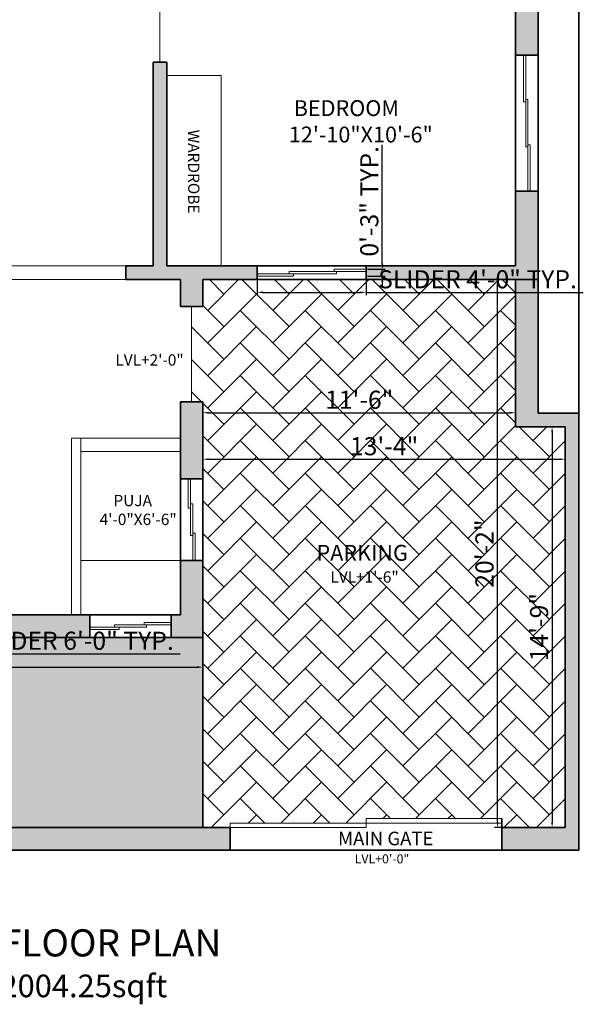
# Model space of a CAD drawing. Units: inches. Extents: x 3491 to 6898, y 1360 to 2019.
# Tile 2 of 9: x 3825 to 4074, y 1360 to 1795. Entities that reach past the tile are written whole.
import ezdxf

# ---------------------------------------------------------------- set-up
doc = ezdxf.new("R2010")
doc.units = ezdxf.units.IN
for name, color, linetype, lineweight in [('A-ANNO-DIMS', 2, 'Continuous', 18), ('A-ANNO-TEXT', 7, 'Continuous', 18), ('A-ANNO-TITL', 7, 'Continuous', 30), ('A-AREA-IDEN', 7, 'Continuous', 18), ('A-DOOR', 4, 'Continuous', 18), ('A-FLOR-CASE', 8, 'Continuous', 18), ('A-FLOR-PATT', 252, 'Continuous', 13), ('A-GLAZ', 5, 'Continuous', 18), ('A-WALL', 7, 'Continuous', 35), ('A-WALL-PATT', 8, 'Continuous', 13)]:
    doc.layers.add(name, color=color, linetype=linetype, lineweight=lineweight)
doc.layers.add('A-WALL-OPEN', color=251, linetype='Continuous', lineweight=13, true_color=0x636466)
doc.styles.get("Standard").update_dxf_attribs({"font": 'arial.ttf'})
doc.dimstyles.new('ISO-25', dxfattribs={"dimtxt": 8, "dimasz": 2.5, "dimexe": 1.25, "dimexo": 0.625, "dimtad": 1, "dimdec": 1, "dimlunit": 3, "dimtxsty": 'Standard', "dimcen": 2.5, "dimclrt": 1, "dimadec": 0, "dimazin": 0, "dimtfac": 1, "dimtdec": 1, "dimtmove": 0, "dimatfit": 3, "dimfxl": 1, "dimarcsym": 0})

# ---------------------------------------------------------------- blocks, each defined once
blk = doc.blocks.new('*D8')
at = {"layer": 'A-ANNO-DIMS', "color": 0, "lineweight": -2, "transparency": 16777216}
for p, q in [((3906.13, 1521.74), (3906.13, 1507.99)), ((3674.13, 1515.52), (3674.13, 1507.99)), ((3676.63, 1509.24), (3903.63, 1509.24))]:
    blk.add_line(p, q, dxfattribs=at)
at = {"layer": 'A-ANNO-DIMS', "color": 0, "transparency": 16777216}
for points in [[(3676.63, 1509.66), (3676.63, 1508.83), (3674.13, 1509.24)], [(3903.63, 1509.66), (3903.63, 1508.83), (3906.13, 1509.24)]]:
    blk.add_solid(points, dxfattribs=at)
at = {"layer": 'Defpoints', "color": 0, "transparency": 16777216}
for p in [(3906.13, 1522.37), (3674.13, 1516.15), (3906.13, 1509.24)]:
    blk.add_point(p, dxfattribs=at)
at = {"layer": 'A-ANNO-DIMS', "color": 0, "transparency": 16777216, "insert": (3790.13, 1513.95), "char_height": 8, "attachment_point": 5}
blk.add_mtext('19\'-4"', dxfattribs=at)
blk = doc.blocks.new('*D25')
at = {"layer": 'A-ANNO-DIMS', "color": 0, "lineweight": -2, "transparency": 16777216}
for p, q in [((3906.13, 1617.55), (3906.13, 1622.78)), ((3908.63, 1621.53), (4041.63, 1621.53)), ((4044.13, 1617.55), (4044.13, 1622.78))]:
    blk.add_line(p, q, dxfattribs=at)
at = {"layer": 'A-ANNO-DIMS', "color": 0, "transparency": 16777216}
for points in [[(3908.63, 1621.95), (3908.63, 1621.12), (3906.13, 1621.53)], [(4041.63, 1621.95), (4041.63, 1621.12), (4044.13, 1621.53)]]:
    blk.add_solid(points, dxfattribs=at)
at = {"layer": 'Defpoints', "color": 0, "transparency": 16777216}
for p in [(4044.13, 1621.53), (3906.13, 1616.92), (4044.13, 1616.92)]:
    blk.add_point(p, dxfattribs=at)
at = {"layer": 'A-ANNO-DIMS', "color": 0, "transparency": 16777216, "insert": (3975.13, 1626.24), "char_height": 8, "attachment_point": 5}
blk.add_mtext('11\'-6"', dxfattribs=at)
blk = doc.blocks.new('*D26')
at = {"layer": 'A-ANNO-DIMS', "color": 0, "lineweight": -2, "transparency": 16777216}
for p, q in [((3906.13, 1601.63), (3906.13, 1602.25)), ((3908.63, 1601), (4063.63, 1601)), ((4066.13, 1601.63), (4066.13, 1602.25))]:
    blk.add_line(p, q, dxfattribs=at)
at = {"layer": 'A-ANNO-DIMS', "color": 0, "transparency": 16777216}
for points in [[(3908.63, 1601.42), (3908.63, 1600.59), (3906.13, 1601)], [(4063.63, 1601.42), (4063.63, 1600.59), (4066.13, 1601)]]:
    blk.add_solid(points, dxfattribs=at)
at = {"layer": 'Defpoints', "color": 0, "transparency": 16777216}
for p in [(3906.13, 1601), (4066.13, 1601), (4066.13, 1601)]:
    blk.add_point(p, dxfattribs=at)
at = {"layer": 'A-ANNO-DIMS', "color": 0, "transparency": 16777216, "insert": (3986.13, 1605.72), "char_height": 8, "attachment_point": 5}
blk.add_mtext('13\'-4"', dxfattribs=at)
blk = doc.blocks.new('*D27')
at = {"layer": 'A-ANNO-DIMS', "color": 0, "lineweight": -2, "transparency": 16777216}
for p, q in [((4065.51, 1615.37), (4059.06, 1615.37)), ((4060.31, 1612.87), (4060.31, 1440.87)), ((4065.51, 1438.37), (4059.06, 1438.37))]:
    blk.add_line(p, q, dxfattribs=at)
at = {"layer": 'A-ANNO-DIMS', "color": 0, "transparency": 16777216}
for points in [[(4059.89, 1612.87), (4060.73, 1612.87), (4060.31, 1615.37)], [(4059.89, 1440.87), (4060.73, 1440.87), (4060.31, 1438.37)]]:
    blk.add_solid(points, dxfattribs=at)
at = {"layer": 'Defpoints', "color": 0, "transparency": 16777216}
for p in [(4066.13, 1615.37), (4060.31, 1438.37), (4066.13, 1438.37)]:
    blk.add_point(p, dxfattribs=at)
at = {"layer": 'A-ANNO-DIMS', "color": 0, "transparency": 16777216, "insert": (4055.6, 1526.87), "char_height": 8, "attachment_point": 5, "rotation": 90}
blk.add_mtext('14\'-9"', dxfattribs=at)
blk = doc.blocks.new('*D28')
at = {"layer": 'A-ANNO-DIMS', "color": 0, "lineweight": -2, "transparency": 16777216}
for p, q in [((4043.51, 1680.37), (4034.93, 1680.37)), ((4036.18, 1440.87), (4036.18, 1677.87)), ((4044.55, 1438.37), (4034.93, 1438.37))]:
    blk.add_line(p, q, dxfattribs=at)
at = {"layer": 'A-ANNO-DIMS', "color": 0, "transparency": 16777216}
for points in [[(4035.76, 1677.87), (4036.6, 1677.87), (4036.18, 1680.37)], [(4035.76, 1440.87), (4036.6, 1440.87), (4036.18, 1438.37)]]:
    blk.add_solid(points, dxfattribs=at)
at = {"layer": 'Defpoints', "color": 0, "transparency": 16777216}
for p in [(4036.18, 1680.37), (4044.13, 1680.37), (4045.17, 1438.37)]:
    blk.add_point(p, dxfattribs=at)
at = {"layer": 'A-ANNO-DIMS', "color": 0, "transparency": 16777216, "insert": (4031.47, 1559.37), "char_height": 8, "attachment_point": 5, "rotation": 90}
blk.add_mtext('20\'-2"', dxfattribs=at)
blk = doc.blocks.new('WIN-SLIDER-48IN')
for p, q in [((35, 1), (0, 1)), ((48, 2), (14, 2)), ((14, 2), (14, 1)), ((16, 1), (16, 0)), ((34, 3), (34, 2)), ((48, 3), (34, 3)), ((35, 2), (35, 1)), ((16, 0), (0, 0))]:
    blk.add_line(p, q)
blk = doc.blocks.new('WIN-SLIDER-36IN')
for p, q in [((25, 1), (0, 1)), ((13, 0), (0, 0)), ((36, 2), (11, 2)), ((11, 2), (11, 1)), ((13, 1), (13, 0)), ((24, 3), (24, 2)), ((36, 3), (24, 3)), ((25, 2), (25, 1))]:
    blk.add_line(p, q)
blk = doc.blocks.new('WIN-SLIDER-60IN')
for p, q in [((0, 39.5), (0, 60)), ((1, 19.5), (1, 60)), ((1, 39.5), (0, 39.5)), ((2, 40.5), (1, 40.5)), ((2, 0), (2, 40.5)), ((2, 19.5), (1, 19.5)), ((3, 20.5), (2, 20.5)), ((3, 0), (3, 20.5))]:
    blk.add_line(p, q)
blk = doc.blocks.new('PUJA-ALCOVE-48X78')
for p, q in [((0, 78), (0, 0)), ((48, 78), (0, 78)), ((4, 78), (4, 0)), ((48, 72), (4, 72)), ((48, 24), (4, 24))]:
    blk.add_line(p, q)
blk = doc.blocks.new('WARDROBE-84X24')
for q in [(0, 84), (24, 0)]:
    blk.add_line((24, 84), q)
blk = doc.blocks.new('*D112')
at = {"layer": 'A-ANNO-DIMS', "color": 0, "lineweight": -2, "transparency": 16777216}
for p, q in [((3930.13, 1681.24), (3930.13, 1673.42)), ((3978.13, 1681.24), (3978.13, 1673.42)), ((3932.63, 1674.67), (3975.63, 1674.67)), ((3978.13, 1674.67), (4074.08, 1674.67))]:
    blk.add_line(p, q, dxfattribs=at)
at = {"layer": 'A-ANNO-DIMS', "color": 0, "transparency": 16777216}
for points in [[(3932.63, 1675.08), (3932.63, 1674.25), (3930.13, 1674.67)], [(3975.63, 1675.08), (3975.63, 1674.25), (3978.13, 1674.67)]]:
    blk.add_solid(points, dxfattribs=at)
at = {"layer": 'Defpoints', "color": 0, "transparency": 16777216}
for p in [(3930.13, 1681.87), (3978.13, 1681.87), (3978.13, 1674.67)]:
    blk.add_point(p, dxfattribs=at)
at = {"layer": 'A-ANNO-DIMS', "color": 1, "transparency": 16777216, "insert": (4027.36, 1679.43), "char_height": 8, "attachment_point": 5}
blk.add_mtext('SLIDER 4\'-0" TYP.', dxfattribs=at)
blk = doc.blocks.new('*D113')
at = {"layer": 'A-ANNO-DIMS', "color": 0, "lineweight": -2, "transparency": 16777216}
for p, q in [((3985.33, 1687.37), (3985.33, 1739.88)), ((3978.76, 1684.87), (3986.58, 1684.87)), ((3985.33, 1681.87), (3985.33, 1684.87)), ((3978.76, 1681.87), (3986.58, 1681.87)), ((3985.33, 1679.37), (3985.33, 1676.87))]:
    blk.add_line(p, q, dxfattribs=at)
at = {"layer": 'A-ANNO-DIMS', "color": 0, "transparency": 16777216}
for points in [[(3984.92, 1687.37), (3985.75, 1687.37), (3985.33, 1684.87)], [(3984.92, 1679.37), (3985.75, 1679.37), (3985.33, 1681.87)]]:
    blk.add_solid(points, dxfattribs=at)
at = {"layer": 'Defpoints', "color": 0, "transparency": 16777216}
for p in [(3978.13, 1684.87), (3985.33, 1684.87), (3978.13, 1681.87)]:
    blk.add_point(p, dxfattribs=at)
at = {"layer": 'A-ANNO-DIMS', "color": 1, "transparency": 16777216, "insert": (3980.62, 1714.87), "char_height": 8, "attachment_point": 5, "rotation": 90}
blk.add_mtext('0\'-3" TYP.', dxfattribs=at)
blk = doc.blocks.new('*D120')
at = {"layer": 'A-ANNO-DIMS', "color": 0, "lineweight": -2, "transparency": 16777216}
for p, q in [((3728.13, 1525.24), (3728.13, 1513.82)), ((3800.13, 1525.24), (3800.13, 1513.82)), ((3730.63, 1515.07), (3797.63, 1515.07)), ((3800.13, 1515.07), (3896.08, 1515.07))]:
    blk.add_line(p, q, dxfattribs=at)
at = {"layer": 'A-ANNO-DIMS', "color": 0, "transparency": 16777216}
for points in [[(3730.63, 1515.48), (3730.63, 1514.65), (3728.13, 1515.07)], [(3797.63, 1515.48), (3797.63, 1514.65), (3800.13, 1515.07)]]:
    blk.add_solid(points, dxfattribs=at)
at = {"layer": 'Defpoints', "color": 0, "transparency": 16777216}
for p in [(3728.13, 1525.87), (3800.13, 1525.87), (3800.13, 1515.07)]:
    blk.add_point(p, dxfattribs=at)
at = {"layer": 'A-ANNO-DIMS', "color": 1, "transparency": 16777216, "insert": (3849.36, 1519.83), "char_height": 8, "attachment_point": 5}
blk.add_mtext('SLIDER 6\'-0" TYP.', dxfattribs=at)

msp = doc.modelspace()

# ---------------------------------------------------------------- hatches: boundary and pattern name
at = {"layer": 'A-FLOR-PATT'}
h = msp.add_hatch(dxfattribs=at)
h.set_pattern_fill('AR-HBONE', color=256, scale=0.1)
h.paths.add_polyline_path([(4038.13, 1442.37), (4038.13, 1438.37), (4066.13, 1438.37), (4066.13, 1615.37), (4044.13, 1615.37), (4044.13, 1680.37), (3906.13, 1680.37), (3906.13, 1668.37), (3901.13, 1668.37), (3901.13, 1626.37), (3906.13, 1626.37), (3906.13, 1438.37), (3918.13, 1438.37), (3918.13, 1440.37), (3978.13, 1440.37), (3978.13, 1442.37)])
h.paths.add_polyline_path([(3958.55, 1617.93), (3991.02, 1617.93), (3991.02, 1634.41), (3958.55, 1634.41)], flags=24)
h.paths.add_polyline_path([(3969.55, 1597.4), (4002.02, 1597.4), (4002.02, 1613.89), (3969.55, 1613.89)], flags=24)
h.paths.add_polyline_path([(4063.92, 1510.28), (4063.92, 1542.75), (4047.43, 1542.75), (4047.43, 1510.28)], flags=24)
h.paths.add_polyline_path([(4039.79, 1543.23), (4039.79, 1575.7), (4023.3, 1575.7), (4023.3, 1543.23)], flags=24)
h.paths.add_polyline_path([(3953.75, 1543.14), (4001.27, 1543.14), (4001.27, 1566.66), (3953.75, 1566.66)], flags=24)
h = msp.add_hatch(dxfattribs=at)
h.set_pattern_fill('ANSI36', color=256, scale=0.5, angle=45)
h.paths.add_polyline_path([(3674.13, 1438.37), (3906.13, 1438.37), (3906.13, 1522.37), (3674.13, 1522.37)])
h.paths.add_polyline_path([(3821.85, 1474.19), (3821.85, 1486.54), (3805.36, 1486.54), (3805.36, 1474.19)], flags=24)
h.paths.add_polyline_path([(3773.55, 1505.64), (3806.02, 1505.64), (3806.02, 1522.12), (3773.55, 1522.12)], flags=24)
h.paths.add_polyline_path([(3741.67, 1455.94), (3796.08, 1455.94), (3796.08, 1491.16), (3741.67, 1491.16)], flags=24)
at = {"layer": 'A-WALL-PATT'}
h = msp.add_hatch(color=256, dxfattribs=at)
h.dxf.hatch_style = 1
h.paths.add_polyline_path([(3856.13, 1532.37), (3800.13, 1532.37), (3800.13, 1522.37), (3856.13, 1522.37)])
h.paths.add_polyline_path([(3906.13, 1626.37), (3896.13, 1626.37), (3896.13, 1592.37), (3906.13, 1592.37)])
h.paths.add_polyline_path([(3906.13, 1556.37), (3896.13, 1556.37), (3896.13, 1532.37), (3892.13, 1532.37), (3892.13, 1522.37), (3906.13, 1522.37)])
h.paths.add_polyline_path([(3728.13, 1532.37), (3680.13, 1532.37), (3680.13, 1680.37), (3794.13, 1680.37), (3794.13, 1686.37), (3674.13, 1686.37), (3674.13, 1532.37), (3656.16, 1532.37), (3656.16, 1522.37), (3728.13, 1522.37)])
h.paths.add_polyline_path([(3608.16, 1532.37), (3542.13, 1532.37), (3542.13, 1580.4), (3532.13, 1580.4), (3532.13, 1428.37), (3674.13, 1428.37), (3674.13, 1438.37), (3542.13, 1438.37), (3542.13, 1522.37), (3608.16, 1522.37)])
h.paths.add_polyline_path([(3542.13, 1722.37), (3620.13, 1722.37), (3620.13, 1782.37), (3614.13, 1782.37), (3614.13, 1728.37), (3542.13, 1728.37), (3542.13, 1770.37), (3532.13, 1770.37), (3532.13, 1628.4), (3542.13, 1628.4)])
h.paths.add_polyline_path([(3906.13, 1680.37), (3930.13, 1680.37), (3930.13, 1686.37), (3890.13, 1686.37), (3890.13, 1776.37), (3884.13, 1776.37), (3884.13, 1686.37), (3872.13, 1686.37), (3872.13, 1680.37), (3896.13, 1680.37), (3896.13, 1668.37), (3906.13, 1668.37)])
h.paths.add_polyline_path([(4054.13, 1719.37), (4044.13, 1719.37), (4044.13, 1686.37), (3978.13, 1686.37), (3978.13, 1680.37), (4054.13, 1680.37)])
h.paths.add_polyline_path([(4054.13, 1857.37), (4044.13, 1857.37), (4044.13, 1818.37), (3884.13, 1818.37), (3884.13, 1812.37), (4044.13, 1812.37), (4044.13, 1779.37), (4054.13, 1779.37)])
h.paths.add_polyline_path([(3848.13, 1872.37), (3842.13, 1872.37), (3842.13, 1818.37), (3782.13, 1818.37), (3782.13, 1902.37), (3800.13, 1902.37), (3800.13, 1908.37), (3758.13, 1908.37), (3758.13, 1902.37), (3776.13, 1902.37), (3776.13, 1818.37), (3716.13, 1818.37), (3716.13, 1872.37), (3710.13, 1872.37), (3710.13, 1812.37), (3848.13, 1812.37)])
h.paths.add_polyline_path([(3542.13, 1857.37), (3532.13, 1857.37), (3532.13, 1794.37), (3542.13, 1794.37), (3542.13, 1812.37), (3674.13, 1812.37), (3674.13, 1818.37), (3542.13, 1818.37)])
h.paths.add_polyline_path([(3542.13, 1962.37), (3710.13, 1962.37), (3710.13, 1938.37), (3716.13, 1938.37), (3716.13, 1962.37), (3842.13, 1962.37), (3842.13, 1938.37), (3848.13, 1938.37), (3848.13, 1962.37), (4044.13, 1962.37), (4044.13, 1923.37), (4054.13, 1923.37), (4054.13, 1972.37), (3532.13, 1972.37), (3532.13, 1923.37), (3542.13, 1923.37)])
h.paths.add_polyline_path([(3734.13, 1908.37), (3710.13, 1908.37), (3710.13, 1902.37), (3734.13, 1902.37)])
h.paths.add_polyline_path([(3848.13, 1908.37), (3824.13, 1908.37), (3824.13, 1902.37), (3848.13, 1902.37)], flags=17)
h = msp.add_hatch(color=256, dxfattribs=at)
h.dxf.hatch_style = 1
h.paths.add_polyline_path([(3918.13, 1438.37), (3674.13, 1438.37), (3674.13, 1428.37), (3918.13, 1428.37)])
h.paths.add_polyline_path([(4072.13, 1621.37), (4054.13, 1621.37), (4054.13, 1680.37), (4044.13, 1680.37), (4044.13, 1615.37), (4066.13, 1615.37), (4066.13, 1438.37), (4038.13, 1438.37), (4038.13, 1428.37), (4072.13, 1428.37)])

# ---------------------------------------------------------------- linework, layer by layer
at = {"layer": 'A-DOOR'}
for p, q in [((3887.13, 1776.37), (3887.13, 1812.37)), ((3901.13, 1626.37), (3901.13, 1668.37)), ((4038.13, 1440.37), (3918.13, 1440.37)), ((3918.13, 1440.37), (3918.13, 1438.37)), ((3978.13, 1438.37), (3978.13, 1442.37)), ((3978.13, 1442.37), (4038.13, 1442.37)), ((3978.13, 1438.37), (3918.13, 1438.37))]:
    msp.add_line(p, q, dxfattribs=at)
at = {"layer": 'A-WALL'}
for p, q in [((4054.13, 1972.37), (4054.13, 1621.37)), ((4072.13, 1428.37), (4072.13, 1972.37)), ((4044.13, 1812.37), (4044.13, 1686.37)), ((4054.13, 1779.37), (4044.13, 1779.37)), ((3884.13, 1776.37), (3884.13, 1686.37)), ((3890.13, 1776.37), (3884.13, 1776.37)), ((3890.13, 1776.37), (3890.13, 1686.37)), ((4054.13, 1719.37), (4044.13, 1719.37)), ((3884.13, 1686.37), (3872.13, 1686.37)), ((3872.13, 1686.37), (3872.13, 1680.37)), ((4044.13, 1686.37), (3890.13, 1686.37)), ((3930.13, 1686.37), (3930.13, 1680.37)), ((3978.13, 1686.37), (3978.13, 1680.37)), ((3896.13, 1680.37), (3872.13, 1680.37)), ((3896.13, 1680.37), (3896.13, 1668.37)), ((4054.13, 1680.37), (3906.13, 1680.37)), ((3906.13, 1680.37), (3906.13, 1668.37)), ((4044.13, 1680.37), (4044.13, 1615.37)), ((3906.13, 1668.37), (3896.13, 1668.37)), ((3896.13, 1626.37), (3896.13, 1532.37)), ((3906.13, 1626.37), (3896.13, 1626.37)), ((3906.13, 1626.37), (3906.13, 1438.37)), ((4072.13, 1621.37), (4054.13, 1621.37)), ((4066.13, 1615.37), (4044.13, 1615.37)), ((4066.13, 1438.37), (4066.13, 1615.37)), ((3906.13, 1592.37), (3896.13, 1592.37)), ((3906.13, 1556.37), (3896.13, 1556.37)), ((3896.13, 1532.37), (3680.13, 1532.37)), ((3856.13, 1532.37), (3856.13, 1522.37)), ((3892.13, 1532.37), (3892.13, 1522.37)), ((3906.13, 1522.37), (3542.13, 1522.37)), ((4038.13, 1442.37), (4038.13, 1428.37)), ((3542.13, 1438.37), (3918.13, 1438.37)), ((3918.13, 1438.37), (3918.13, 1428.37)), ((4038.13, 1438.37), (4066.13, 1438.37)), ((3532.13, 1428.37), (4072.13, 1428.37))]:
    msp.add_line(p, q, dxfattribs=at)
at = {"layer": 'A-WALL-OPEN'}
for p, q in [((3872.13, 1686.37), (3794.13, 1686.37)), ((3794.13, 1680.37), (3872.13, 1680.37))]:
    msp.add_line(p, q, dxfattribs=at)

# ---------------------------------------------------------------- block references
at = {"layer": 'A-FLOR-CASE'}
for name, p in [('WARDROBE-84X24', (3890.13, 1686.37)), ('PUJA-ALCOVE-48X78', (3848.13, 1532.37))]:
    msp.add_blockref(name, p, dxfattribs=at)
at = {"layer": 'A-GLAZ'}
for name, p in [('WIN-SLIDER-60IN', (4047.63, 1719.37)), ('WIN-SLIDER-48IN', (3930.13, 1681.87)), ('WIN-SLIDER-36IN', (3856.13, 1525.87))]:
    msp.add_blockref(name, p, dxfattribs=at)
at = {"layer": 'A-GLAZ', "rotation": 270}
msp.add_blockref('WIN-SLIDER-36IN', (3899.63, 1592.37), dxfattribs=at)

# ---------------------------------------------------------------- texts
at = {"layer": 'A-ANNO-TEXT', "insert": (3904.58, 1746.53), "char_height": 5, "attachment_point": 1, "rotation": 270}
msp.add_mtext_dynamic_manual_height_columns('WARDROBE', width=86.9528, gutter_width=12.5, heights=[0], dxfattribs=at)
at = {"layer": 'A-ANNO-TEXT', "attachment_point": 1}
for s, width, insert, char_height in [('{LVL+2\'-0"}', 33.0959, (3867.44, 1647.35), 5), ('{\\H0.85714x;MAIN GATE}\\P{\\H0.57143x;      LVL+0\'-0"}', 121.6144, (3965.78, 1436.56), 7)]:
    msp.add_mtext_dynamic_manual_height_columns(s, width=width, gutter_width=12.5, heights=[0], dxfattribs=dict(at, insert=insert, char_height=char_height))
at = {"layer": 'A-ANNO-TITL', "insert": (3744.49, 1393.48), "char_height": 12, "attachment_point": 1}
msp.add_mtext_dynamic_manual_height_columns('GROUND FLOOR PLAN\\P{\\H0.83333x;SLAB AREA 2004.25sqft}', width=285.9409, gutter_width=12.5, heights=[0], dxfattribs=at)
at = {"layer": 'A-AREA-IDEN', "attachment_point": 1}
for s, width, insert, char_height in [(' BEDROOM\\P12\'-10"X10\'-6"', 121.6144, (3944.05, 1759.53), 7), ('    PUJA\\P4\'-0"X6\'-6"', 33.0959, (3860.48, 1585.28), 5), ('PARKING\\P{\\H0.71429x;    LVL+1\'-6"}', 121.6144, (3956.26, 1563.18), 7)]:
    msp.add_mtext_dynamic_manual_height_columns(s, width=width, gutter_width=12.5, heights=[0], dxfattribs=dict(at, insert=insert, char_height=char_height))

# ---------------------------------------------------------------- dimensions: what is measured, and where the dimension line sits
at = {"layer": 'A-ANNO-DIMS'}
dim = msp.add_linear_dim(base=(3985.33, 1684.87), p1=(3978.13, 1681.87), p2=(3978.13, 1684.87), angle=90, text='<> TYP.', dimstyle='ISO-25', override={"dimdec": 1, "dimlfac": 1, "dimrnd": 0, "dimzin": 1, "dimdsep": 46, "dimlunit": 4, "dimfrac": 2}, dxfattribs=at)
dim.commit()
dim.dimension.update_dxf_attribs({"geometry": '*D113', "text_midpoint": (3980.62, 1714.87)})
for base, p1, p2, picture, middle in [((3978.13, 1674.67), (3930.13, 1681.87), (3978.13, 1681.87), '*D112', (4027.36, 1679.43)), ((3800.13, 1515.07), (3728.13, 1525.87), (3800.13, 1525.87), '*D120', (3849.36, 1519.83))]:
    dim = msp.add_linear_dim(base=base, p1=p1, p2=p2, text='SLIDER <> TYP.', dimstyle='ISO-25', override={"dimdec": 1, "dimlfac": 1, "dimrnd": 0, "dimzin": 1, "dimdsep": 46, "dimlunit": 4, "dimfrac": 2}, dxfattribs=at)
    dim.commit()
    dim.dimension.update_dxf_attribs({"geometry": picture, "text_midpoint": middle})
for base, p1, p2, picture, middle in [((4036.18, 1680.37), (4045.17, 1438.37), (4044.13, 1680.37), '*D28', (4031.47, 1559.37)), ((4060.31, 1438.37), (4066.13, 1615.37), (4066.13, 1438.37), '*D27', (4055.6, 1526.87))]:
    dim = msp.add_linear_dim(base=base, p1=p1, p2=p2, angle=90, dimstyle='ISO-25', override={"dimclrd": 0, "dimclre": 0, "dimclrt": 0}, dxfattribs=at)
    dim.commit()
    dim.dimension.update_dxf_attribs({"geometry": picture, "text_midpoint": middle})
for base, p1, p2, picture, middle in [((4044.13, 1621.53), (3906.13, 1616.92), (4044.13, 1616.92), '*D25', (3975.13, 1626.24)), ((4066.13, 1601), (3906.13, 1601), (4066.13, 1601), '*D26', (3986.13, 1605.72)), ((3906.13, 1509.24), (3674.13, 1516.15), (3906.13, 1522.37), '*D8', (3790.13, 1513.95))]:
    dim = msp.add_linear_dim(base=base, p1=p1, p2=p2, dimstyle='ISO-25', override={"dimclrd": 0, "dimclre": 0, "dimclrt": 0}, dxfattribs=at)
    dim.commit()
    dim.dimension.update_dxf_attribs({"geometry": picture, "text_midpoint": middle})

doc.saveas('drawing.dxf')
